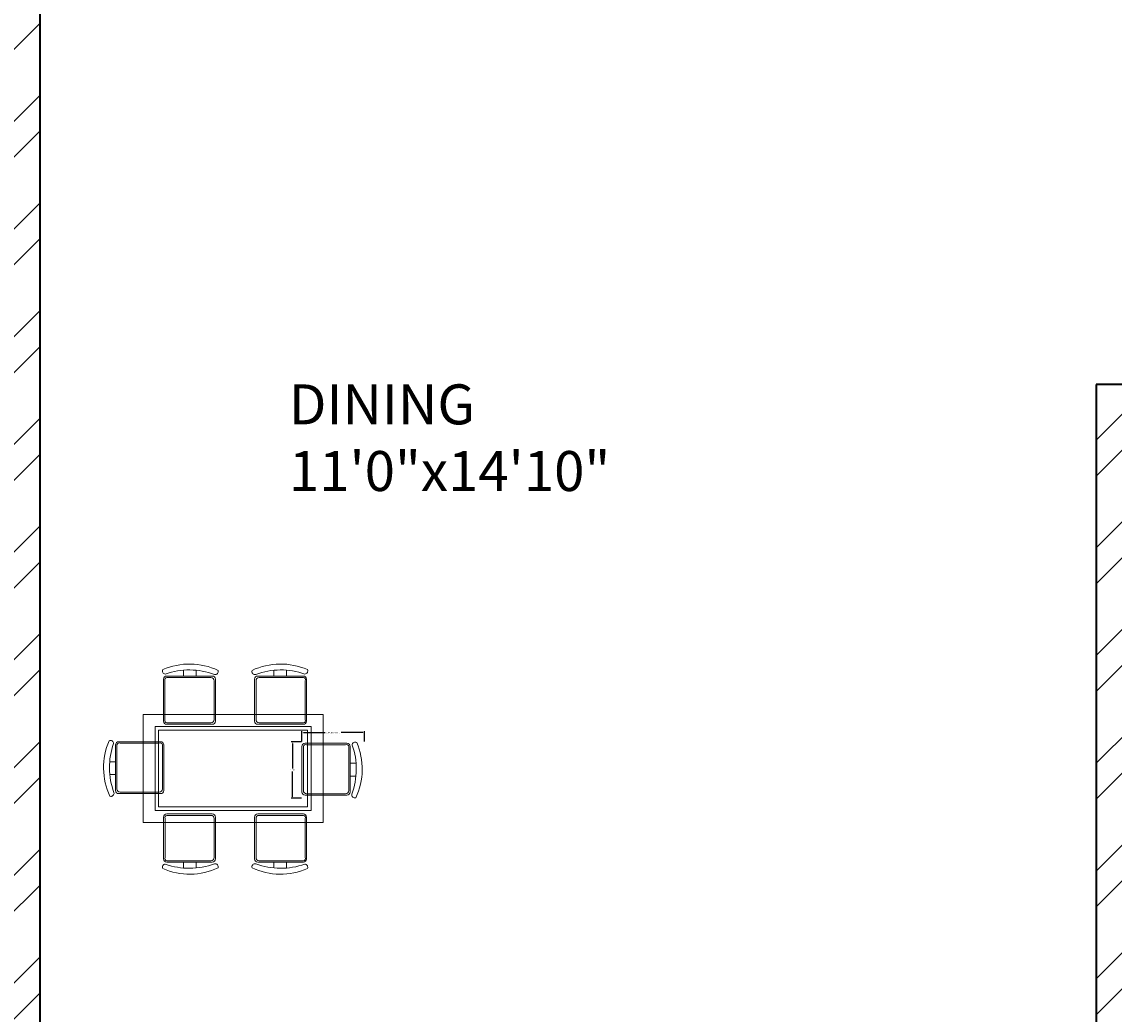
# Model space of a CAD drawing. Units: inches. Extents: x 1962 to 2771, y 1245 to 2660.
# Tile 110 of 114: x 2374 to 2510, y 2180 to 2304. Entities that reach past the tile are written whole.
import ezdxf

# ---------------------------------------------------------------- set-up
doc = ezdxf.new("R2010")
doc.units = ezdxf.units.IN
for name, color, linetype, lineweight in [('A-ANNO-DIMS', 2, 'Continuous', 18), ('A-AREA-IDEN', 7, 'Continuous', 18), ('A-FURN', 8, 'Continuous', 13), ('A-WALL', 7, 'Continuous', 35), ('A-WALL-PATT', 252, 'Continuous', 13)]:
    doc.layers.add(name, color=color, linetype=linetype, lineweight=lineweight)
doc.styles.get("Standard").update_dxf_attribs({"font": 'arial.ttf'})
doc.dimstyles.get("Standard").update_dxf_attribs({"dimtxt": 0.18, "dimasz": 0.18, "dimexe": 0.18, "dimexo": 0.0625, "dimgap": 0.09, "dimtad": 0, "dimtih": 1, "dimtoh": 1, "dimdec": 4, "dimzin": 0, "dimdsep": 46, "dimtxsty": 'Standard', "dimcen": 0.09, "dimadec": 0, "dimazin": 0, "dimtfac": 1, "dimtdec": 4, "dimtofl": 0, "dimtmove": 0, "dimatfit": 3, "dimfxl": 1, "dimtolj": 1, "dimtzin": 0, "dimarcsym": 0})

# ---------------------------------------------------------------- blocks, each defined once
blk = doc.blocks.new('DINING-TABLE')
for points in [[(0, 13.51), (22.52, 13.51), (22.52, 0), (0, 0)], [(0, 13.51), (22.52, 13.51), (22.52, 0), (0, 0)], [(1.5, 12.01), (21.02, 12.01), (21.02, 1.5), (1.5, 1.5)], [(1.5, 12.01), (21.02, 12.01), (21.02, 1.5), (1.5, 1.5)], [(1.95, 11.56), (20.57, 11.56), (20.57, 1.95), (1.95, 1.95)], [(1.95, 11.56), (20.57, 11.56), (20.57, 1.95), (1.95, 1.95)]]:
    blk.add_lwpolyline(points, close=True)
blk = doc.blocks.new('DINING-CHAIR-B')
for points in [[(6.03, 6.44, 0.414214), (5.63, 6.84), (0.4, 6.84, 0.414214), (0, 6.44), (0, 0.74, 0.414214), (0.4, 0.35), (5.63, 0.35, 0.414214), (6.03, 0.74), (6.03, 6.44)], [(6.03, 6.44, 0.414214), (5.63, 6.84), (0.4, 6.84, 0.414214), (0, 6.44), (0, 0.74, 0.414214), (0.4, 0.35), (5.63, 0.35, 0.414214), (6.03, 0.74), (6.03, 6.44)], [(6.28, 6.62, -0.175809), (6.23, 0.48, 0.578392), (6.74, 0.02, 0.214524), (6.84, 6.94, 0.552014), (6.28, 6.62, -0.065079)], [(6.28, 6.62, -0.175809), (6.23, 0.48, 0.578392), (6.74, 0.02, 0.214524), (6.84, 6.94, 0.552014), (6.28, 6.62, -0.065079)], [(6.03, 2.74), (6.75, 2.74, -0.064759)], [(6.03, 2.74), (6.75, 2.74, -0.064759)]]:
    blk.add_lwpolyline(points, format="xyb")
blk.add_lwpolyline([(5.85, 6.44), (5.85, 0.92, -0.414214), (5.45, 0.53), (0.58, 0.53, -0.414214), (0.18, 0.92), (0.18, 6.44, -0.512069), (0.58, 6.66), (5.45, 6.66, -0.512069)], format="xyb", close=True)
blk.add_lwpolyline([(5.85, 6.44), (5.85, 0.92, -0.414214), (5.45, 0.53), (0.58, 0.53, -0.414214), (0.18, 0.92), (0.18, 6.44, -0.512069), (0.58, 6.66), (5.45, 6.66, -0.512069)], format="xyb", close=True)
blk.add_lwpolyline([(6.77, 4.34), (6.03, 4.34)])
blk.add_lwpolyline([(6.77, 4.34), (6.03, 4.34)])
blk = doc.blocks.new('DINING-CHAIR-C')
for points in [[(6.24, 1.5), (0.55, 1.5, -0.414214), (0.15, 1.9), (0.15, 7.14, -0.414214), (0.55, 7.53), (6.24, 7.53, -0.414214), (6.64, 7.14), (6.64, 1.9, -0.414214), (6.24, 1.5)], [(6.24, 1.5), (0.55, 1.5, -0.414214), (0.15, 1.9), (0.15, 7.13, -0.414214), (0.55, 7.53), (6.24, 7.53, -0.414214), (6.64, 7.13), (6.64, 1.9, -0.414214), (6.24, 1.5)], [(4.24, 1.5), (4.24, 0.78, 0.064759)], [(4.24, 1.5), (4.24, 0.78, 0.064759)], [(6.5, 1.3, -0.578392), (6.97, 0.79, -0.214524), (0.04, 0.7, -0.552014), (0.37, 1.25, 0.175809), (6.5, 1.3)], [(6.5, 1.3, -0.578392), (6.97, 0.79, -0.214524), (0.04, 0.7, -0.552014), (0.37, 1.25, 0.175809), (6.5, 1.3)]]:
    blk.add_lwpolyline(points, format="xyb")
blk.add_lwpolyline([(0.55, 1.68), (6.06, 1.68, 0.414214), (6.46, 2.08), (6.46, 6.96, 0.414214), (6.06, 7.35), (0.55, 7.35, 0.512069), (0.33, 6.96), (0.33, 2.08, 0.512069)], format="xyb", close=True)
blk.add_lwpolyline([(0.55, 1.68), (6.06, 1.68, 0.414214), (6.46, 2.08), (6.46, 6.96, 0.414214), (6.06, 7.35), (0.55, 7.35, 0.512069), (0.33, 6.96), (0.33, 2.08, 0.512069)], format="xyb", close=True)
blk.add_lwpolyline([(2.65, 0.77), (2.65, 1.5)])
blk.add_lwpolyline([(2.65, 0.77), (2.65, 1.5)])
blk = doc.blocks.new('*D36')
at = {"layer": 'A-ANNO-DIMS', "color": 0, "lineweight": -2, "transparency": 16777216}
for p, q in [((2408.56, 2214.19), (2408.56, 2215.48)), ((2416.36, 2214.19), (2416.36, 2215.48)), ((2408.74, 2215.3), (2411.46, 2215.3)), ((2416.18, 2215.3), (2413.46, 2215.3))]:
    blk.add_line(p, q, dxfattribs=at)
at = {"layer": 'A-ANNO-DIMS', "color": 0, "transparency": 16777216}
for points in [[(2408.74, 2215.33), (2408.74, 2215.27), (2408.56, 2215.3)], [(2416.18, 2215.33), (2416.18, 2215.27), (2416.36, 2215.3)]]:
    blk.add_solid(points, dxfattribs=at)
at = {"layer": 'Defpoints', "color": 0, "transparency": 16777216}
for p in [(2408.56, 2214.13), (2416.36, 2215.3), (2416.36, 2214.13)]:
    blk.add_point(p, dxfattribs=at)
at = {"layer": 'A-ANNO-DIMS', "color": 0, "transparency": 16777216, "insert": (2412.46, 2215.3), "char_height": 0.18, "attachment_point": 5}
blk.add_mtext('\\A1;CHAIR B 8 TYP.', dxfattribs=at)
blk = doc.blocks.new('*D37')
at = {"layer": 'A-ANNO-DIMS', "color": 0, "lineweight": -2, "transparency": 16777216}
for p, q in [((2408.5, 2214.13), (2407.21, 2214.13)), ((2407.39, 2213.95), (2407.39, 2210.8)), ((2407.39, 2207.28), (2407.39, 2210.44)), ((2408.5, 2207.1), (2407.21, 2207.1))]:
    blk.add_line(p, q, dxfattribs=at)
at = {"layer": 'A-ANNO-DIMS', "color": 0, "transparency": 16777216}
for points in [[(2407.36, 2213.95), (2407.42, 2213.95), (2407.39, 2214.13)], [(2407.36, 2207.28), (2407.42, 2207.28), (2407.39, 2207.1)]]:
    blk.add_solid(points, dxfattribs=at)
at = {"layer": 'Defpoints', "color": 0, "transparency": 16777216}
for p in [(2407.39, 2214.13), (2408.56, 2214.13), (2408.56, 2207.1)]:
    blk.add_point(p, dxfattribs=at)
at = {"layer": 'A-ANNO-DIMS', "color": 0, "transparency": 16777216, "insert": (2407.39, 2210.62), "char_height": 0.18, "attachment_point": 5}
blk.add_mtext('\\A1;7 TYP.', dxfattribs=at)
blk = doc.blocks.new('*D40')
at = {"layer": 'A-ANNO-DIMS', "color": 0, "lineweight": -2, "transparency": 16777216}
for p, q in [((2072.02, 2033.91), (2072.02, 2583.47)), ((2072.2, 2583.29), (2366.02, 2583.29)), ((2660.63, 2583.29), (2366.81, 2583.29)), ((2660.81, 2524.41), (2660.81, 2583.47))]:
    blk.add_line(p, q, dxfattribs=at)
at = {"layer": 'A-ANNO-DIMS', "color": 0, "transparency": 16777216}
for points in [[(2072.2, 2583.32), (2072.2, 2583.26), (2072.02, 2583.29)], [(2660.63, 2583.32), (2660.63, 2583.26), (2660.81, 2583.29)]]:
    blk.add_solid(points, dxfattribs=at)
at = {"layer": 'Defpoints', "color": 0, "transparency": 16777216}
for p in [(2660.81, 2583.29), (2660.81, 2524.34), (2072.02, 2033.84)]:
    blk.add_point(p, dxfattribs=at)
at = {"layer": 'A-ANNO-DIMS', "color": 0, "transparency": 16777216, "insert": (2366.41, 2583.29), "char_height": 0.18, "attachment_point": 5}
blk.add_mtext('\\A1;588.8', dxfattribs=at)

msp = doc.modelspace()

# ---------------------------------------------------------------- hatches: boundary and pattern name
at = {"layer": 'A-WALL-PATT'}
h = msp.add_hatch(dxfattribs=at)
h.set_pattern_fill('ANSI32', color=256)
h.paths.add_polyline_path([(2090.8074, 2467.3437), (2141.6481, 2467.3437), (2141.6481, 2469.5937), (2141.6481, 2471.8437), (2086.3074, 2471.8437), (2086.3074, 2422.5333), (2090.8074, 2422.5333)])
h.paths.add_polyline_path([(2282.7664, 2471.8437), (2204.8982, 2471.8437), (2204.8982, 2467.3437), (2234.8074, 2467.3437), (2234.8074, 2311.3437), (2228.7492, 2311.3437), (2228.7492, 2306.8437), (2234.8074, 2306.8437), (2331.9227, 2306.8437), (2331.9227, 2309.0937), (2331.9227, 2311.3437), (2239.3074, 2311.3437), (2239.3074, 2467.3437), (2282.7664, 2467.3437), (2282.7664, 2469.5937)])
h.paths.add_polyline_path([(2471.4531, 2519.8437), (2552.011, 2519.8437), (2564.3996, 2519.8437), (2564.3996, 2511.1389), (2568.8996, 2511.1389), (2568.8996, 2524.3437), (2466.9531, 2524.3437), (2466.9531, 2471.8437), (2450.0749, 2471.8437), (2446.4672, 2471.8437), (2446.4672, 2467.3437), (2450.0749, 2467.3437), (2475.9988, 2467.3437), (2475.9988, 2469.5937), (2475.9988, 2471.8437), (2471.4531, 2471.8437)])
h.paths.add_polyline_path([(2575.2231, 2469.5937), (2575.2231, 2471.8437), (2568.8996, 2471.8437), (2568.8996, 2487.1389), (2564.3996, 2487.1389), (2564.3996, 2471.8437), (2556.511, 2471.8437), (2499.2904, 2471.8437), (2499.2904, 2467.3437), (2507.8074, 2467.3437), (2507.8074, 2311.3437), (2414.863, 2311.3437), (2414.863, 2306.8437), (2512.3074, 2306.8437), (2517.0114, 2306.8437), (2517.0114, 2309.0937), (2517.0114, 2311.3437), (2512.3074, 2311.3437), (2512.3074, 2467.3437), (2575.2231, 2467.3437)])
h.paths.add_polyline_path([(2660.8074, 2471.8437), (2600.9602, 2471.8437), (2600.9602, 2467.3437), (2656.3074, 2467.3437), (2656.3074, 2432.5704), (2660.8074, 2432.5704)])
h.paths.add_polyline_path([(2660.8074, 2372.5704), (2656.3074, 2372.5704), (2656.3074, 2311.3437), (2600.276, 2311.3437), (2600.276, 2309.0937), (2600.276, 2306.8437), (2656.3074, 2306.8437), (2656.3074, 2296.2593), (2660.8074, 2296.2593)])
h.paths.add_polyline_path([(2572.3074, 2306.8437), (2577.1385, 2306.8437), (2577.1385, 2311.3437), (2551.082, 2311.3437), (2551.082, 2306.8437), (2567.8074, 2306.8437), (2567.8074, 2258.8437), (2540.0574, 2258.8437), (2540.0574, 2256.5937), (2540.0574, 2254.3437), (2567.8074, 2254.3437), (2656.3074, 2254.3437), (2656.3074, 2236.9085), (2660.8074, 2236.9085), (2660.8074, 2272.2593), (2656.3074, 2272.2593), (2656.3074, 2258.8437), (2572.3074, 2258.8437)])
h.paths.add_polyline_path([(2512.3074, 2254.3437), (2518.8716, 2254.3437), (2518.8716, 2256.5937), (2518.8716, 2258.8437), (2507.8074, 2258.8437), (2507.8074, 2177.8437), (2567.8074, 2177.8437), (2567.8074, 2172.9628), (2572.3074, 2172.9628), (2572.3074, 2177.8437), (2656.3074, 2177.8437), (2656.3074, 2166.4846), (2660.8074, 2166.4846), (2660.8074, 2200.9085), (2656.3074, 2200.9085), (2656.3074, 2182.3437), (2512.3074, 2182.3437)])
h.paths.add_polyline_path([(2656.3074, 2129.8437), (2572.3074, 2129.8437), (2572.3074, 2150.3044), (2570.0574, 2150.3044), (2567.8074, 2150.3044), (2567.8074, 2129.8437), (2507.8074, 2129.8437), (2507.8074, 2116.3027), (2510.0574, 2116.3027), (2512.3074, 2116.3027), (2512.3074, 2125.3437), (2567.8074, 2125.3437), (2572.3074, 2125.3437), (2656.3074, 2125.3437)])
h.paths.add_polyline_path([(2090.8074, 2362.5333), (2086.3074, 2362.5333), (2086.3074, 2298.6242), (2090.8074, 2298.6242), (2090.8074, 2306.8437), (2174.8074, 2306.8437), (2174.8074, 2286.4178), (2179.3074, 2286.4178), (2179.3074, 2306.8437), (2192.8641, 2306.8437), (2192.8641, 2309.0937), (2192.8641, 2311.3437), (2090.8074, 2311.3437)])
h.paths.add_polyline_path([(2209.156, 2258.8437), (2179.3074, 2258.8437), (2179.3074, 2263.2236), (2177.0574, 2263.2236), (2174.8074, 2263.2236), (2174.8074, 2258.8437), (2090.8074, 2258.8437), (2090.8074, 2274.6242), (2086.3074, 2274.6242), (2086.3074, 2238.2967), (2088.5574, 2238.2967), (2090.8074, 2238.2967), (2090.8074, 2254.3437), (2209.156, 2254.3437)])
h.paths.add_polyline_path([(2090.8074, 2177.8437), (2234.8074, 2177.8437), (2234.8074, 2173.1428), (2239.3074, 2173.1428), (2239.3074, 2258.8437), (2230.8442, 2258.8437), (2230.8442, 2256.5937), (2230.8442, 2254.3437), (2234.8074, 2254.3437), (2234.8074, 2182.3437), (2090.8074, 2182.3437), (2090.8074, 2202.2967), (2086.3074, 2202.2967), (2086.3074, 2140.0389), (2090.8074, 2140.0389)])
h.paths.add_polyline_path([(2090.8074, 2080.0389), (2086.3074, 2080.0389), (2086.3074, 2033.8437), (2090.8074, 2033.8437)], flags=17)
h.paths.add_polyline_path([(2244.9405, 2033.8437), (2239.3074, 2033.8437), (2239.3074, 2142.0665), (2237.2592, 2142.0665), (2234.8074, 2142.0665), (2234.8074, 2033.8437), (2090.8074, 2033.8437), (2076.5204, 2033.8437), (2072.0204, 2033.8437), (2072.0204, 2000.4493), (2076.5204, 2000.4493), (2076.5204, 2029.3437), (2090.8074, 2029.3437), (2244.9405, 2029.3437), (2244.9405, 2031.5937)])
h.paths.add_polyline_path([(2234.8074, 1933.3437), (2076.5204, 1933.3437), (2076.5204, 1952.4493), (2074.2704, 1952.4493), (2072.0204, 1952.4493), (2072.0204, 1933.3437), (2072.0204, 1928.8437), (2234.8074, 1928.8437)])
h.paths.add_polyline_path([(2090.8074, 1928.8437), (2086.3074, 1928.8437), (2086.3074, 1906.5013), (2090.8074, 1906.5013)])
h.paths.add_polyline_path([(2090.8074, 1846.5013), (2086.3074, 1846.5013), (2086.3074, 1769.9917), (2088.5574, 1769.9917), (2090.8074, 1769.9917), (2090.8074, 1780.3437), (2234.8074, 1780.3437), (2234.8074, 1708.3437), (2230.3764, 1708.3437), (2230.3764, 1703.8437), (2239.3074, 1703.8437), (2239.3074, 1792.6669), (2237.0574, 1792.6669), (2234.8074, 1792.6669), (2234.8074, 1784.8437), (2090.8074, 1784.8437)])
h.paths.add_polyline_path([(2239.3074, 1928.8437), (2244.9405, 1928.8437), (2244.9405, 1931.0937), (2244.9405, 1933.3437), (2234.8074, 1933.3437), (2234.8074, 1928.8437), (2234.8074, 1825.5949), (2239.3074, 1825.5949)])
h.paths.add_polyline_path([(2148.0425, 1649.0937), (2148.0425, 1651.3437), (2090.8074, 1651.3437), (2090.8074, 1646.8437), (2148.0425, 1646.8437)], flags=0)
h.paths.add_polyline_path([(2207.5601, 1708.3437), (2090.8074, 1708.3437), (2090.8074, 1703.8437), (2174.8074, 1703.8437), (2174.8074, 1651.3437), (2170.4457, 1651.3437), (2170.4457, 1646.8437), (2195.9924, 1646.8437), (2195.9924, 1649.0937), (2195.9924, 1651.3437), (2179.3074, 1651.3437), (2179.3074, 1703.8437), (2207.5601, 1703.8437), (2207.5601, 1706.0937)])
h.paths.add_polyline_path([(2090.8074, 1733.9917), (2086.3074, 1733.9917), (2086.3074, 1696.1032), (2088.5574, 1696.1032), (2090.8074, 1696.1032)])
h.paths.add_polyline_path([(2090.8074, 1672.1032), (2086.3074, 1672.1032), (2086.3074, 1600.3335), (2090.8074, 1600.3335)])
h.paths.add_polyline_path([(2090.8074, 1540.3335), (2086.3074, 1540.3335), (2086.3074, 1486.3437), (2139.6766, 1486.3437), (2139.6766, 1490.8437), (2090.8074, 1490.8437)])
h.paths.add_polyline_path([(2302.3876, 1490.8437), (2239.3074, 1490.8437), (2239.3074, 1646.8437), (2335.9994, 1646.8437), (2335.9994, 1651.3437), (2229.884, 1651.3437), (2229.884, 1646.8437), (2234.8074, 1646.8437), (2234.8074, 1490.8437), (2202.7103, 1490.8437), (2202.7103, 1488.5937), (2202.7103, 1486.3437), (2275.0699, 1486.3437), (2275.0699, 1475.772), (2279.5699, 1475.772), (2279.5699, 1486.3437), (2302.3876, 1486.3437)])
h.paths.add_polyline_path([(2279.5699, 1451.772), (2275.0699, 1451.772), (2275.0699, 1438.3437), (2174.8074, 1438.3437), (2174.8074, 1486.3437), (2179.7922, 1486.3437), (2179.7922, 1490.8437), (2163.3585, 1490.8437), (2163.3585, 1488.5937), (2163.3585, 1486.3437), (2170.3074, 1486.3437), (2170.3074, 1433.8437), (2279.5699, 1433.8437)])
h.paths.add_polyline_path([(2427.2363, 1490.8437), (2375.8074, 1490.8437), (2375.8074, 1646.8437), (2381.6401, 1646.8437), (2381.6401, 1651.3437), (2365.887, 1651.3437), (2365.887, 1649.0937), (2365.887, 1646.8437), (2371.3074, 1646.8437), (2371.3074, 1490.8437), (2327.5627, 1490.8437), (2327.5627, 1488.5937), (2327.5627, 1486.3437), (2371.3074, 1486.3437), (2371.3074, 1433.8437), (2375.8074, 1433.8437), (2375.8074, 1486.3437), (2427.2363, 1486.3437)])
h.paths.add_polyline_path([(2512.3074, 1646.8437), (2519.4351, 1646.8437), (2519.4351, 1649.0937), (2519.4351, 1651.3437), (2507.8074, 1651.3437), (2416.0063, 1651.3437), (2416.0063, 1649.0937), (2416.0063, 1646.8437), (2507.8074, 1646.8437), (2507.8074, 1490.8437), (2497.0532, 1490.8437), (2497.0532, 1488.5937), (2497.0532, 1486.3437), (2574.9344, 1486.3437), (2574.9344, 1476.0181), (2579.4344, 1476.0181), (2579.4344, 1486.3437), (2584.4872, 1486.3437), (2584.3074, 1490.8437), (2512.3074, 1490.8437)])
h.paths.add_polyline_path([(2470.5091, 1486.3437), (2473.9767, 1486.3437), (2473.9767, 1490.8437), (2449.6605, 1490.8437), (2449.6605, 1488.5937), (2449.6605, 1486.3437), (2466.0091, 1486.3437), (2466.0091, 1433.8437), (2470.5091, 1433.8437), (2579.4344, 1433.8437), (2579.4344, 1452.0181), (2574.9344, 1452.0181), (2574.9344, 1438.3437), (2554.5091, 1438.3437), (2470.5091, 1438.3437)])
h.paths.add_polyline_path([(2656.3074, 1490.8437), (2611.86, 1490.8437), (2611.86, 1486.3437), (2656.3074, 1486.3437)])
h.paths.add_polyline_path([(2660.8074, 1532.7007), (2658.5574, 1532.7007), (2656.3074, 1532.7007), (2656.3074, 1486.3437), (2660.8074, 1486.3437)])
h.paths.add_polyline_path([(2660.8074, 1664.9663), (2656.3074, 1664.9663), (2656.3074, 1651.3437), (2602.2313, 1651.3437), (2602.2313, 1646.8437), (2656.3074, 1646.8437), (2656.3074, 1592.7007), (2660.8074, 1592.7007)])
h.paths.add_polyline_path([(2660.8074, 1724.5221), (2656.3074, 1724.5221), (2656.3074, 1703.8437), (2542.4725, 1703.8437), (2542.4725, 1699.3437), (2567.8074, 1699.3437), (2567.8074, 1651.3437), (2552.7766, 1651.3437), (2552.7766, 1649.0937), (2552.7766, 1646.8437), (2577.2878, 1646.8437), (2577.2878, 1649.0937), (2577.2878, 1651.3437), (2572.3074, 1651.3437), (2572.3074, 1699.3437), (2656.3074, 1699.3437), (2656.3074, 1688.9663), (2660.8074, 1688.9663)])
h.paths.add_polyline_path([(2660.8074, 1880.6524), (2656.3074, 1880.6524), (2656.3074, 1832.8437), (2512.3074, 1832.8437), (2512.3074, 1837.8959), (2507.8074, 1837.8959), (2507.8074, 1828.3437), (2567.8074, 1828.3437), (2567.8074, 1804.3437), (2572.3074, 1804.3437), (2572.3074, 1828.3437), (2656.3074, 1828.3437), (2656.3074, 1818.6778), (2660.8074, 1818.6778)])
h.paths.add_polyline_path([(2660.8074, 1794.6778), (2656.3074, 1794.6778), (2656.3074, 1780.3437), (2572.3074, 1780.3437), (2572.3074, 1783.0303), (2570.0574, 1783.0303), (2567.8074, 1783.0303), (2567.8074, 1780.3437), (2507.8074, 1780.3437), (2507.8074, 1699.3437), (2517.8858, 1699.3437), (2517.8858, 1701.5937), (2517.8858, 1703.8437), (2512.3074, 1703.8437), (2512.3074, 1775.8437), (2656.3074, 1775.8437), (2656.3074, 1760.5221), (2660.8074, 1760.5221)])
h.paths.add_polyline_path([(2660.8074, 1981.3437), (2660.8074, 2020.2808), (2658.5574, 2020.2808), (2656.3074, 2020.2808), (2656.3074, 1981.3437), (2512.3074, 1981.3437), (2512.3074, 2086.6996), (2507.8074, 2086.6996), (2507.8074, 1981.3437), (2375.8074, 1981.3437), (2375.8074, 1986.8505), (2373.5574, 1986.8505), (2371.3074, 1986.8505), (2371.3074, 1973.2607), (2375.8074, 1973.2607), (2375.8074, 1976.8437), (2507.8074, 1976.8437), (2507.8074, 1865.4281), (2510.0574, 1865.4281), (2512.3074, 1865.4281), (2512.3074, 1976.8437), (2660.8074, 1976.8437)])
h.paths.add_polyline_path([(2375.8074, 1940.297), (2373.5574, 1940.297), (2371.3074, 1940.297), (2371.3074, 1933.3437), (2278.4434, 1933.3437), (2278.4434, 1928.8437), (2371.3074, 1928.8437), (2371.3074, 1651.3437), (2375.8074, 1651.3437)])
h.paths.add_polyline_path([(2660.8074, 1976.8437), (2656.3074, 1976.8437), (2656.3074, 1940.6524), (2660.8074, 1940.6524)], flags=17)
h.paths.add_polyline_path([(2660.8074, 2142.4846), (2656.3074, 2142.4846), (2656.3074, 2080.2808), (2660.8074, 2080.2808)])
h.paths.add_polyline_path([(2381.4189, 2311.3437), (2375.8074, 2311.3437), (2375.8074, 2467.3437), (2424.7242, 2467.3437), (2424.7242, 2469.5937), (2424.7242, 2471.8437), (2375.8074, 2471.8437), (2375.8074, 2524.3437), (2371.3074, 2524.3437), (2371.3074, 2471.8437), (2307.2097, 2471.8437), (2307.2097, 2467.3437), (2371.3074, 2467.3437), (2371.3074, 2311.3437), (2366.8901, 2311.3437), (2366.8901, 2306.8437), (2371.3074, 2306.8437), (2371.3074, 2033.8437), (2279.6589, 2033.8437), (2279.6589, 2029.3437), (2371.3074, 2029.3437), (2371.3074, 2014.2598), (2375.8074, 2014.2598), (2375.8074, 2306.8437), (2381.4189, 2306.8437)])
h.paths.add_polyline_path([(2263.3074, 2524.3437), (2170.3074, 2524.3437), (2170.3074, 2519.8437), (2170.3074, 2471.8437), (2165.0312, 2471.8437), (2165.0312, 2467.3437), (2179.6721, 2467.3437), (2179.6721, 2469.5161), (2179.6721, 2471.8437), (2174.8074, 2471.8437), (2174.8074, 2519.8437), (2258.8074, 2519.8437), (2258.8074, 2511.6436), (2263.3074, 2511.6436)])
h.paths.add_polyline_path([(2245.0232, 1361.4123), (2492.9468, 1361.4123), (2492.9468, 1398.505), (2245.0232, 1398.505)], flags=9)
h.paths.add_polyline_path([(2388.1434, 2086.6936), (2425.0704, 2086.6936), (2425.0704, 2105.3509), (2388.1434, 2105.3509)], flags=9)
h.paths.add_polyline_path([(2404.922, 2242.6744), (2445.7337, 2242.6744), (2445.7337, 2261.3318), (2404.922, 2261.3318)], flags=9)
h.paths.add_polyline_path([(2269.4107, 2156.7935), (2306.3378, 2156.7935), (2306.3378, 2175.4508), (2269.4107, 2175.4508)], flags=9)
h.paths.add_polyline_path([(2269.3277, 2233.4343), (2306.2547, 2233.4343), (2306.2547, 2252.0917), (2269.3277, 2252.0917)], flags=9)
h.paths.add_polyline_path([(2431.6052, 2320.6922), (2470.4456, 2320.6922), (2470.4456, 2339.3495), (2431.6052, 2339.3495)], flags=25)
h.paths.add_polyline_path([(2249.6902, 2315.7608), (2288.5306, 2315.7608), (2288.5306, 2334.4182), (2249.6902, 2334.4182)], flags=25)
h.paths.add_polyline_path([(2096.9301, 2314.3181), (2135.7704, 2314.3181), (2135.7704, 2332.9755), (2096.9301, 2332.9755)], flags=25)
h.paths.add_polyline_path([(2134.3475, 2285.7089), (2161.4655, 2285.7089), (2161.4655, 2304.3662), (2134.3475, 2304.3662)], flags=9)
h.paths.add_polyline_path([(2126.5155, 2209.4076), (2159.9227, 2209.4076), (2159.9227, 2228.065), (2126.5155, 2228.065)], flags=25)
h.paths.add_polyline_path([(2110.5753, 2141.5299), (2149.4157, 2141.5299), (2149.4157, 2160.1872), (2110.5753, 2160.1872)], flags=25)
h.paths.add_polyline_path([(2249.8618, 1968.3317), (2286.3966, 1968.3317), (2286.3966, 1986.989), (2249.8618, 1986.989)], flags=9)
h.paths.add_polyline_path([(2395.9507, 1777.0051), (2436.7624, 1777.0051), (2436.7624, 1795.6625), (2395.9507, 1795.6625)], flags=9)
h.paths.add_polyline_path([(2398.5259, 1888.5651), (2435.0062, 1888.5651), (2435.0062, 1907.2224), (2398.5259, 1907.2224)], flags=25)
h.paths.add_polyline_path([(2259.3506, 1728.3559), (2296.2776, 1728.3559), (2296.2776, 1747.0132), (2259.3506, 1747.0132)], flags=9)
h.paths.add_polyline_path([(2271.3698, 1845.268), (2308.2968, 1845.268), (2308.2968, 1863.9253), (2271.3698, 1863.9253)], flags=9)
h.paths.add_polyline_path([(2120.9355, 1786.3027), (2159.7759, 1786.3027), (2159.7759, 1804.9601), (2120.9355, 1804.9601)], flags=25)
h.paths.add_polyline_path([(2121.3164, 1732.1043), (2154.7236, 1732.1043), (2154.7236, 1750.7616), (2121.3164, 1750.7616)], flags=25)
h.paths.add_polyline_path([(2118.3706, 1678.8997), (2147.5282, 1678.8997), (2147.5282, 1697.557), (2118.3706, 1697.557)], flags=25)
h.paths.add_polyline_path([(2385.9227, 1493.557), (2424.763, 1493.557), (2424.763, 1512.2143), (2385.9227, 1512.2143)], flags=25)
h.paths.add_polyline_path([(2248.7058, 1500.0256), (2287.5462, 1500.0256), (2287.5462, 1518.6829), (2248.7058, 1518.6829)], flags=25)
h.paths.add_polyline_path([(2104.1669, 1617.3771), (2143.0073, 1617.3771), (2143.0073, 1636.0344), (2104.1669, 1636.0344)], flags=9)
h.paths.add_polyline_path([(2096.0714, 1447.8824), (2137.3845, 1447.8824), (2137.3845, 1458.1859), (2096.0714, 1458.1859)], flags=9)
h.paths.add_polyline_path([(2180.6114, 1440.325), (2209.7689, 1440.325), (2209.7689, 1458.9823), (2180.6114, 1458.9823)], flags=25)
h.paths.add_polyline_path([(2316.1698, 1447.9637), (2357.4829, 1447.9637), (2357.4829, 1458.2673), (2316.1698, 1458.2673)], flags=9)
h.paths.add_polyline_path([(2397.6187, 1447.9637), (2438.9318, 1447.9637), (2438.9318, 1458.2673), (2397.6187, 1458.2673)], flags=9)
h.paths.add_polyline_path([(2473.0778, 1439.5953), (2502.2354, 1439.5953), (2502.2354, 1458.2527), (2473.0778, 1458.2527)], flags=25)
h.paths.add_polyline_path([(2589.7027, 1447.8819), (2631.0158, 1447.8819), (2631.0158, 1458.1855), (2589.7027, 1458.1855)], flags=9)
h.paths.add_polyline_path([(2522.4009, 1497.5285), (2561.2413, 1497.5285), (2561.2413, 1516.1859), (2522.4009, 1516.1859)], flags=25)
h.paths.add_polyline_path([(2579.6565, 1671.3482), (2608.8141, 1671.3482), (2608.8141, 1690.0056), (2579.6565, 1690.0056)], flags=25)
h.paths.add_polyline_path([(2544.7038, 1725.5064), (2578.1111, 1725.5064), (2578.1111, 1744.1637), (2544.7038, 1744.1637)], flags=25)
h.paths.add_polyline_path([(2578.1191, 1807.472), (2607.2766, 1807.472), (2607.2766, 1826.1293), (2578.1191, 1826.1293)], flags=25)
h.paths.add_polyline_path([(2595.0614, 1835.1839), (2633.9018, 1835.1839), (2633.9018, 1853.8413), (2595.0614, 1853.8413)], flags=25)
h.paths.add_polyline_path([(2567.0097, 2097.7035), (2605.8501, 2097.7035), (2605.8501, 2116.3609), (2567.0097, 2116.3609)], flags=9)
h.paths.add_polyline_path([(2586.644, 2134.6454), (2615.8015, 2134.6454), (2615.8015, 2153.3027), (2586.644, 2153.3027)], flags=9)
h.paths.add_polyline_path([(2544.6185, 2212.6783), (2578.0258, 2212.6783), (2578.0258, 2231.3356), (2544.6185, 2231.3356)], flags=25)
h.paths.add_polyline_path([(2577.0273, 2256.9023), (2606.1849, 2256.9023), (2606.1849, 2275.5597), (2577.0273, 2275.5597)], flags=24)
h.paths.add_polyline_path([(2605.2683, 2315.2821), (2644.1087, 2315.2821), (2644.1087, 2333.9395), (2605.2683, 2333.9395)], flags=25)
h.paths.add_polyline_path([(2583.1244, 2496.1815), (2624.4375, 2496.1815), (2624.4375, 2506.4851), (2583.1244, 2506.4851)], flags=9)
h.paths.add_polyline_path([(2474.761, 2497.0823), (2503.9185, 2497.0823), (2503.9185, 2515.7397), (2474.761, 2515.7397)], flags=25)
h.paths.add_polyline_path([(2387.5787, 2494.2563), (2428.902, 2494.2563), (2428.902, 2504.5598), (2387.5787, 2504.5598)], flags=9)
h.paths.add_polyline_path([(2300.1657, 2500.1564), (2341.4788, 2500.1564), (2341.4788, 2510.46), (2300.1657, 2510.46)], flags=25)
h.paths.add_polyline_path([(2176.8589, 2497.5843), (2206.0165, 2497.5843), (2206.0165, 2516.2416), (2176.8589, 2516.2416)], flags=25)
h.paths.add_polyline_path([(2097.4668, 2494.9762), (2138.7799, 2494.9762), (2138.7799, 2505.2798), (2097.4668, 2505.2798)], flags=9)

# ---------------------------------------------------------------- linework, layer by layer
at = {"layer": 'A-FURN'}
for points in [[(2391.4856, 2222.6194, -0.17580919), (2397.6195, 2222.573, 0.57839206), (2398.0842, 2223.0839, 0.21452438), (2391.1603, 2223.1768, 0.55201397), (2391.4856, 2222.6194, -0.06507904)], [(2391.4856, 2222.6192, -0.17580919), (2397.6195, 2222.5727, 0.57839206), (2398.0842, 2223.0837, 0.21452438), (2391.1603, 2223.1766, 0.55201397), (2391.4856, 2222.6192, -0.06507904)], [(2402.7834, 2222.573, -0.57839206), (2402.3187, 2223.0839, -0.21452438), (2409.2425, 2223.1768, -0.55201397), (2408.9172, 2222.6194, 0.1758092), (2402.7834, 2222.573)], [(2402.7834, 2222.5727, -0.57839206), (2402.3187, 2223.0837, -0.21452438), (2409.2425, 2223.1766, -0.55201397), (2408.9173, 2222.6192, 0.1758092), (2402.7834, 2222.5727)], [(2397.3592, 2222.3732), (2391.6648, 2222.3732, 0.41421356), (2391.2664, 2221.9749), (2391.2664, 2216.7389, 0.41421356), (2391.6648, 2216.3405), (2397.3592, 2216.3405, 0.41421356), (2397.7576, 2216.7389), (2397.7576, 2221.9749, 0.41421356), (2397.3592, 2222.3732)], [(2397.3592, 2222.373), (2391.6648, 2222.373, 0.41421356), (2391.2664, 2221.9746), (2391.2664, 2216.7387, 0.41421356), (2391.6648, 2216.3403), (2397.3592, 2216.3403, 0.41421356), (2397.7576, 2216.7387), (2397.7576, 2221.9746, 0.41421356), (2397.3592, 2222.373)], [(2395.359, 2222.3732), (2395.359, 2223.0934, -0.06475861)], [(2395.3591, 2222.373), (2395.3591, 2223.0932, -0.06475861)], [(2408.7381, 2222.3732, -0.41421356), (2409.1365, 2221.9749), (2409.1365, 2216.7389, -0.41421356), (2408.7381, 2216.3405), (2403.0436, 2216.3405, -0.41421356), (2402.6452, 2216.7389), (2402.6452, 2221.9749, -0.41421356), (2403.0436, 2222.3732), (2408.7381, 2222.3732)], [(2408.7381, 2222.373, -0.41421356), (2409.1365, 2221.9746), (2409.1365, 2216.7387, -0.41421356), (2408.7381, 2216.3403), (2403.0436, 2216.3403, -0.41421356), (2402.6452, 2216.7387), (2402.6452, 2221.9746, -0.41421356), (2403.0436, 2222.373), (2408.7381, 2222.373)], [(2405.0438, 2222.3732), (2405.0438, 2223.0934, 0.06475861)], [(2405.0438, 2222.373), (2405.0438, 2223.0932, 0.06475861)], [(2385.0684, 2207.8071, -0.57839206), (2384.5574, 2207.3424, -0.21452438), (2384.4645, 2214.2662, -0.55201397), (2385.022, 2213.9409, 0.17580937), (2385.0684, 2207.8071)], [(2385.0684, 2207.8068, -0.57839206), (2384.5575, 2207.3422, -0.21452438), (2384.4646, 2214.266, -0.55201397), (2385.022, 2213.9407, 0.17580937), (2385.0684, 2207.8068)], [(2385.2681, 2213.7618, -0.41421356), (2385.6665, 2214.1602), (2390.9025, 2214.1602, -0.41421356), (2391.3009, 2213.7618), (2391.3009, 2208.0673, -0.41421356), (2390.9025, 2207.6689), (2385.6665, 2207.6689, -0.41421356), (2385.2681, 2208.0673), (2385.2681, 2213.7618)], [(2385.2682, 2213.7615, -0.41421356), (2385.6665, 2214.1599), (2390.9025, 2214.1599, -0.41421356), (2391.3009, 2213.7615), (2391.3009, 2208.0671, -0.41421356), (2390.9025, 2207.6687), (2385.6665, 2207.6687, -0.41421356), (2385.2682, 2208.0671), (2385.2682, 2213.7615)], [(2385.2681, 2210.0675), (2384.548, 2210.0675, 0.06475861)], [(2385.2682, 2210.0673), (2384.548, 2210.0673, 0.06475861)], [(2408.7381, 2199.0981, 0.41421356), (2409.1365, 2199.4965), (2409.1365, 2204.7325, 0.41421356), (2408.7381, 2205.1309), (2403.0436, 2205.1309, 0.41421356), (2402.6452, 2204.7325), (2402.6452, 2199.4965, 0.41421356), (2403.0436, 2199.0981), (2408.7381, 2199.0981)], [(2408.7381, 2199.0979, 0.41421356), (2409.1365, 2199.4963), (2409.1365, 2204.7323, 0.41421356), (2408.7381, 2205.1306), (2403.0436, 2205.1306, 0.41421356), (2402.6452, 2204.7323), (2402.6452, 2199.4963, 0.41421356), (2403.0436, 2199.0979), (2408.7381, 2199.0979)], [(2405.0438, 2199.0981), (2405.0438, 2198.378, -0.06475861)], [(2405.0438, 2199.0979), (2405.0438, 2198.3777, -0.06475861)], [(2408.9172, 2198.852, -0.17580928), (2402.7834, 2198.8984, 0.57839206), (2402.3187, 2198.3874, 0.21452438), (2409.2425, 2198.2945, 0.55201397), (2408.9172, 2198.852, -0.06507904)], [(2408.9173, 2198.8517, -0.17580928), (2402.7834, 2198.8982, 0.57839206), (2402.3187, 2198.3872, 0.21452438), (2409.2425, 2198.2943, 0.55201397), (2408.9173, 2198.8517, -0.06507904)]]:
    msp.add_lwpolyline(points, format="xyb", dxfattribs=at)
for points in [[(2393.7651, 2223.1065), (2393.7651, 2222.3732)], [(2393.7651, 2223.1063), (2393.7651, 2222.373)], [(2406.6378, 2223.1065), (2406.6378, 2222.3732)], [(2406.6378, 2223.1063), (2406.6378, 2222.373)], [(2384.5349, 2211.6615), (2385.2681, 2211.6615)], [(2384.5349, 2211.6612), (2385.2682, 2211.6612)], [(2406.6378, 2198.3649), (2406.6378, 2199.0981)], [(2406.6378, 2198.3646), (2406.6378, 2199.0979)]]:
    msp.add_lwpolyline(points, dxfattribs=at)
for points in [[(2391.6672, 2222.1938), (2397.1798, 2222.1938, -0.41421356), (2397.5781, 2221.7954), (2397.5781, 2216.9184, -0.41421356), (2397.1798, 2216.52), (2391.6672, 2216.52, -0.51206948), (2391.4458, 2216.9184), (2391.4458, 2221.7954, -0.51206948)], [(2391.6672, 2222.1935), (2397.1798, 2222.1935, -0.41421356), (2397.5782, 2221.7951), (2397.5782, 2216.9181, -0.41421356), (2397.1798, 2216.5197), (2391.6672, 2216.5197, -0.51206948), (2391.4459, 2216.9181), (2391.4459, 2221.7951, -0.51206948)], [(2408.7357, 2222.1938), (2403.2231, 2222.1938, 0.41421356), (2402.8247, 2221.7954), (2402.8247, 2216.9184, 0.41421356), (2403.2231, 2216.52), (2408.7357, 2216.52, 0.51206948), (2408.957, 2216.9184), (2408.957, 2221.7954, 0.51206948)], [(2408.7357, 2222.1935), (2403.2231, 2222.1935, 0.41421356), (2402.8247, 2221.7951), (2402.8247, 2216.9181, 0.41421356), (2403.2231, 2216.5197), (2408.7357, 2216.5197, 0.51206948), (2408.957, 2216.9181), (2408.957, 2221.7951, 0.51206948)], [(2385.4476, 2213.7594), (2385.4476, 2208.2468, 0.41421356), (2385.846, 2207.8484), (2390.723, 2207.8484, 0.41421356), (2391.1214, 2208.2468), (2391.1214, 2213.7594, 0.51206948), (2390.723, 2213.9807), (2385.846, 2213.9807, 0.51206948)], [(2385.4476, 2213.7591), (2385.4476, 2208.2466, 0.41421356), (2385.846, 2207.8482), (2390.723, 2207.8482, 0.41421356), (2391.1214, 2208.2466), (2391.1214, 2213.7591, 0.51206948), (2390.723, 2213.9805), (2385.846, 2213.9805, 0.51206948)], [(2408.7357, 2199.2776), (2403.2231, 2199.2776, -0.41421356), (2402.8247, 2199.676), (2402.8247, 2204.553, -0.41421356), (2403.2231, 2204.9514), (2408.7357, 2204.9514, -0.51206948), (2408.957, 2204.553), (2408.957, 2199.676, -0.51206948)], [(2408.7357, 2199.2774), (2403.2231, 2199.2774, -0.41421356), (2402.8247, 2199.6758), (2402.8247, 2204.5528, -0.41421356), (2403.2231, 2204.9512), (2408.7357, 2204.9512, -0.51206948), (2408.957, 2204.5528), (2408.957, 2199.6758, -0.51206948)]]:
    msp.add_lwpolyline(points, format="xyb", close=True, dxfattribs=at)
at = {"layer": 'A-WALL'}
for p, q in [((2375.8074, 2306.8437), (2375.8074, 2014.2598)), ((2507.8074, 2258.8437), (2507.8074, 2177.8437)), ((2518.8716, 2258.8437), (2507.8074, 2258.8437))]:
    msp.add_line(p, q, dxfattribs=at)

# ---------------------------------------------------------------- block references
at = {"layer": 'A-FURN'}
for name, p in [('DINING-TABLE', (2388.7001, 2204.0518)), ('DINING-CHAIR-B', (2408.5593, 2207.128)), ('DINING-CHAIR-C', (2391.1171, 2197.5973))]:
    msp.add_blockref(name, p, dxfattribs=at)

# ---------------------------------------------------------------- texts
at = {"layer": 'A-AREA-IDEN', "insert": (2406.9326, 2258.8437), "char_height": 5, "attachment_point": 1}
msp.add_mtext_dynamic_manual_height_columns('DINING\\P11\'0"x14\'10"', width=207.374791, gutter_width=12.5, heights=[0], dxfattribs=at)

# ---------------------------------------------------------------- dimensions: what is measured, and where the dimension line sits
at = {"layer": 'A-ANNO-DIMS'}
dim = msp.add_linear_dim(base=(2660.8074, 2583.2937), p1=(2072.0204, 2033.8437), p2=(2660.8074, 2524.3437), dimstyle='Standard', override={"dimdec": 1, "dimlfac": 1, "dimrnd": 0, "dimzin": 0, "dimdsep": 46, "dimlunit": 2}, dxfattribs=at)
dim.commit()
dim.dimension.update_dxf_attribs({"geometry": '*D40', "text_midpoint": (2366.4139, 2583.2937)})
dim = msp.add_linear_dim(base=(2416.3563, 2215.3013), p1=(2408.5593, 2214.1318), p2=(2416.3563, 2214.1318), text='CHAIR B <> TYP.', dimstyle='Standard', override={"dimdec": 0, "dimlfac": 1, "dimrnd": 0, "dimzin": 0, "dimdsep": 46, "dimlunit": 2}, dxfattribs=at)
dim.commit()
dim.dimension.update_dxf_attribs({"geometry": '*D36', "text_midpoint": (2412.4578, 2215.3013)})
dim = msp.add_linear_dim(base=(2407.3897, 2214.1318), p1=(2408.5593, 2207.1035), p2=(2408.5593, 2214.1318), angle=90, text='<> TYP.', dimstyle='Standard', override={"dimdec": 0, "dimlfac": 1, "dimrnd": 0, "dimzin": 0, "dimdsep": 46, "dimlunit": 2}, dxfattribs=at)
dim.commit()
dim.dimension.update_dxf_attribs({"geometry": '*D37', "text_midpoint": (2407.3897, 2210.6177)})

doc.saveas('drawing.dxf')
